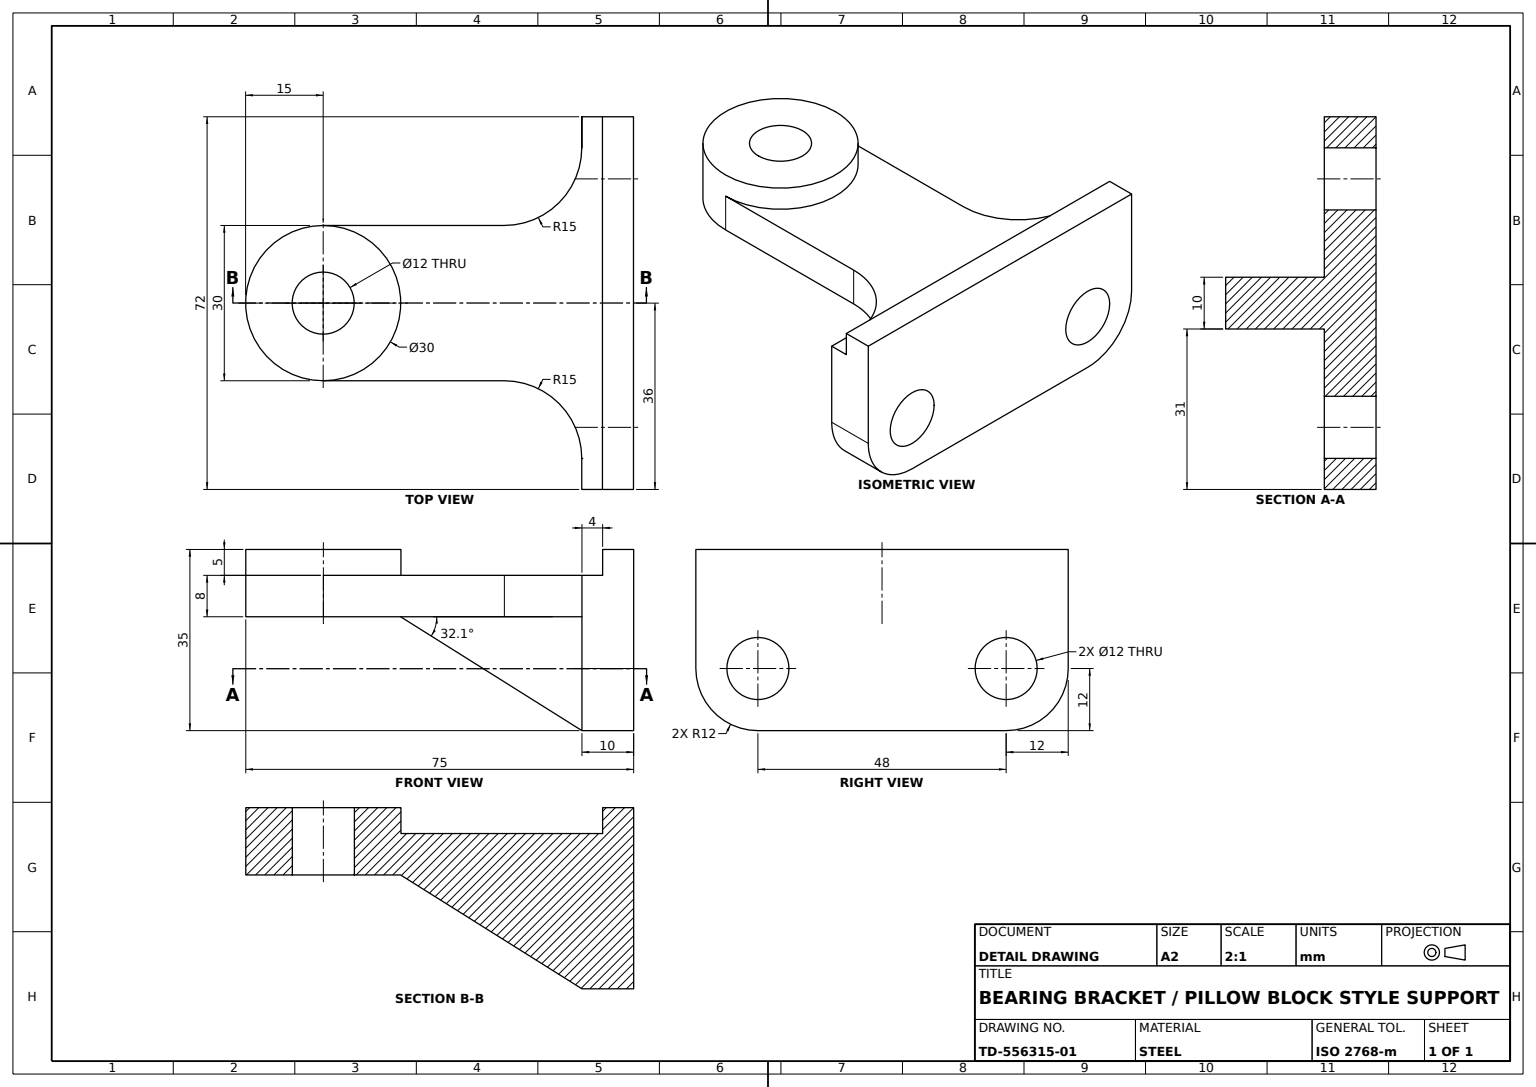
SolidWorks part; units mm, degrees
material "Plain Carbon Steel"
ref_plane "Front Plane" through (0, 0, 0) normal (0, 0, 1) x (1, 0, 0)
ref_plane "Top Plane" through (0, 0, 0) normal (0, 1, 0) x (1, 0, 0)
ref_plane "Right Plane" through (0, 0, 0) normal (1, 0, 0) x (0, 0, -1)
sketch "Base Plate Profile" plane through (0, 0, 0) normal (0, 0, 1) x (1, 0, 0)
  line L0 (0, 0) -> (72, 0)
  line L1 (36, 0) -> (60, 0)
  line L2 (60, 0) -> (60, -23)
  line L3 (36, 0) -> (12, 0)
  line L4 (12, 0) -> (12, -23)
  line L5 (0, 0) -> (0, -23)
  line L6 (72, 0) -> (72, -23)
  line L7 (0, -23) -> (72, -23)
  line L8 (12, -35) -> (60, -35)
  arc A0 (0, -23) -> (12, -35) centre (12, -23) ccw
  arc A1 (60, -35) -> (72, -23) centre (60, -23) ccw
  dimension "D6" = 12
  dimension "D8" = 48
  dimension "D1" = 72
  dimension "D2" = 24
  dimension "D3" = 23
  dimension "D4" = 48
  dimension "D5" = 23
  dimension "D7" = 23
  dimension "D9" = 23
  dimension "D10" = 12
  dimension "D11" = 12
  dimension "D12" = 12
  dimension "D13" = 12
extrude "Base Plate" add sketch "Base Plate Profile" along normal blind 10 contours L4 L7 L2 L0 | L5 L7 L4 L0 | L2 L7 L6 L0 | L8 A1 L7 A0
sketch "Groove Profile 4x5" plane through (72, 0, 0) normal (1, 0, 0) x (0, 0, -1)
  line L0 (-10, 0) -> (-6, 0)
  line L1 (-10, 0) -> (0, 0) construction
  line L2 (-6, 0) -> (-6, -5)
  line L3 (-6, -5) -> (-10, -5)
  line L4 (-10, 0) -> (-10, -23) construction
  line L5 (-10, -5) -> (-10, 0)
  dimension "D1" = 4
  dimension "D2" = 5
extrude "Groove Cut 4x5" cut sketch "Groove Profile 4x5" against normal blind 150
sketch "Arm Profile" plane through (0, -5, 0) normal (0, 1, 0) x (1, 0, 0)
  line L0 (0, -10) -> (0, -6) construction
  line L2 (21, -60) -> (21, -10)
  line L3 (0, -10) -> (72, -10) construction
  line L4 (21, -10) -> (51, -10)
  line L5 (51, -10) -> (51, -60)
  arc A0 (21, -60) -> (51, -60) centre (36, -60) ccw
  dimension "D2" = 30
  dimension "D1" = 50
  dimension "D3" = 30
  dimension "D4" = 50
  dimension "D5" = 21
extrude "Arm" add sketch "Arm Profile" against normal blind 12
sketch "Eye Boss Sketch Ø30" plane through (0, -5, 0) normal (0, 1, 0) x (1, 0, 0)
  circle A0 centre (36, -60) radius 15
  dimension "D1" = 30
extrude "Eye Boss Ø30" add sketch "Eye Boss Sketch Ø30" along normal blind 5
sketch "Arm Relief Profile" plane through (0, -17, 0) normal (0, -1, 0) x (1, 0, 0)
  line L0 (21, 10) -> (21, 60)
  line L1 (51, 10) -> (51, 60)
  line L2 (21, 10) -> (51, 10)
  arc A0 (51, 60) -> (21, 60) centre (36, 60) ccw
extrude "Arm Relief Cut" cut sketch "Arm Relief Profile" against normal blind 4
sketch "Eye Hole Sketch Ø12" plane through (0, -13, 0) normal (0, -1, 0) x (1, 0, 0)
  circle A0 centre (36, 60) radius 6
  dimension "D1" = 12
extrude "Eye Hole Ø12" cut sketch "Eye Hole Sketch Ø12" against normal blind 20
sketch "Upright Rib Profile" plane through (0, -13, 0) normal (0, -1, 0) x (1, 0, 0)
  line L0 (21, 60) -> (21, 10) construction
  line L1 (12, 10) -> (0, 10) construction
  line L2 (51, 10) -> (51, 60) construction
  line L3 (72, 10) -> (60, 10) construction
  line L4 (6, 10) -> (21, 10)
  line L5 (12, 10) -> (60, 10) construction
  line L6 (21, 10) -> (51, 10) construction
  line L7 (21, 10) -> (21, 25)
  line L8 (51, 25) -> (51, 10)
  line L9 (51, 10) -> (66, 10)
  arc A0 (21, 25) -> (6, 10) centre (6, 25) cw
  arc A1 (51, 25) -> (66, 10) centre (66, 25) ccw
  dimension "D1" = 15
extrude "Upright Rib" add sketch "Upright Rib Profile" against normal blind 8
sketch "Cross Hole Sketch Ø12" plane through (0, 0, 10) normal (0, 0, 1) x (1, 0, 0)
  circle A0 centre (12, -23) radius 6
  circle A1 centre (60, -23) radius 6
  dimension "D1" = 12
  dimension "D2" = 12
extrude "Cross Hole Ø12" cut sketch "Cross Hole Sketch Ø12" against normal blind 20
sketch "Upright Web Profile" plane through (0, 0, 0) normal (-1, 0, 0) x (0, 0, 1)
  line L0 (10, -13) -> (45.0718, -13)
  line L1 (60, -13) -> (25, -13) construction
  line L2 (45.0718, -13) -> (10, -35)
  line L3 (10, -35) -> (10, -13)
  dimension "D1" = 35.0718
extrude "Upright Web" add sketch "Upright Web Profile" against normal blind 72
sketch "Web Trim Profile 1" plane through (72, 0, 0) normal (1, 0, 0) x (0, 0, -1)
  line L0 (-45.0718, -13) -> (-10, -13)
  line L1 (-10, -13) -> (-10, -35)
  line L2 (-10, -35) -> (-45.0718, -13)
extrude "Web Trim Cut 1" cut sketch "Web Trim Profile 1" against normal blind 31
sketch "Web Trim Profile 2" plane through (0, 0, 0) normal (-1, 0, 0) x (0, 0, 1)
  line L0 (10, -35) -> (10, -13)
  line L1 (10, -13) -> (45.0718, -13)
  line L2 (45.0718, -13) -> (10, -35)
extrude "Web Trim Cut 2" cut sketch "Web Trim Profile 2" against normal blind 31
